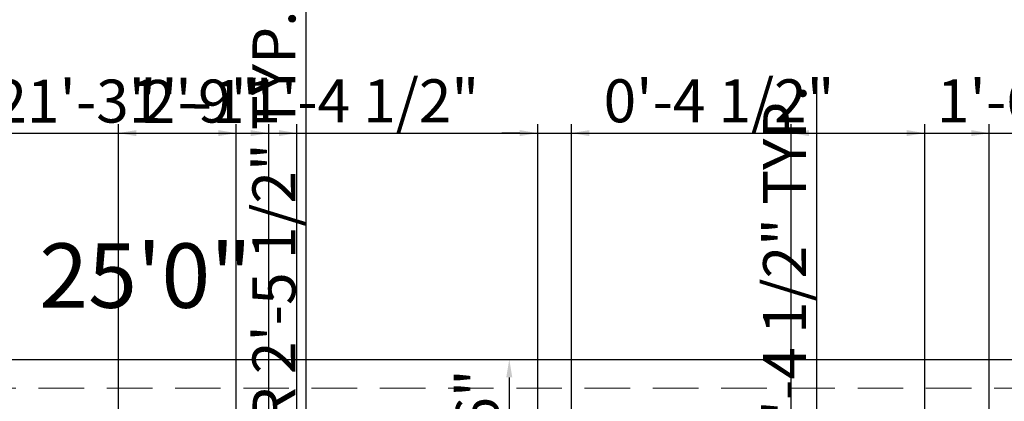
# Model space of a CAD drawing. Units: inches. Extents: x 2656 to 9931, y 1941 to 3068.
# Tile 24 of 46: x 2863 to 3000, y 2636 to 2689. Entities that reach past the tile are written whole.
import ezdxf

# ---------------------------------------------------------------- set-up
doc = ezdxf.new("R2010")
doc.units = ezdxf.units.IN
doc.linetypes.add('DASHED2', pattern=[9.525, 6.35, -3.175])
for name, color, linetype, lineweight in [('A-ANNO-DIMS', 2, 'Continuous', 18), ('A-FLOR-OVHD', 252, 'DASHED2', 13), ('C-PROP', 7, 'Continuous', 25)]:
    doc.layers.add(name, color=color, linetype=linetype, lineweight=lineweight)
doc.styles.get("Standard").update_dxf_attribs({"font": 'arial.ttf'})
doc.dimstyles.new('ISO-25', dxfattribs={"dimtxt": 6, "dimasz": 2.5, "dimexe": 1.25, "dimexo": 0.625, "dimtad": 1, "dimdec": 0, "dimlunit": 3, "dimtxsty": 'Standard', "dimcen": 2.5, "dimadec": 0, "dimazin": 0, "dimtfac": 1, "dimtdec": 0, "dimtmove": 0, "dimatfit": 3, "dimfxl": 1, "dimarcsym": 0})

# ---------------------------------------------------------------- blocks, each defined once
blk = doc.blocks.new('*D2')
at = {"layer": 'A-ANNO-DIMS', "color": 0, "lineweight": -2, "transparency": 16777216}
for p, q in [((2931.82, 2641.6), (2932.44, 2641.6)), ((2931.19, 2639.1), (2931.19, 2626.1)), ((2931.82, 2623.6), (2932.44, 2623.6))]:
    blk.add_line(p, q, dxfattribs=at)
at = {"layer": 'A-ANNO-DIMS', "color": 0, "transparency": 16777216}
for points in [[(2930.77, 2639.1), (2931.61, 2639.1), (2931.19, 2641.6)], [(2930.77, 2626.1), (2931.61, 2626.1), (2931.19, 2623.6)]]:
    blk.add_solid(points, dxfattribs=at)
at = {"layer": 'Defpoints', "color": 0, "transparency": 16777216}
for p in [(2931.19, 2641.6), (2931.19, 2623.6), (2931.19, 2623.6)]:
    blk.add_point(p, dxfattribs=at)
at = {"layer": 'A-ANNO-DIMS', "color": 0, "transparency": 16777216, "insert": (2927.5, 2632.6), "char_height": 6, "attachment_point": 5, "rotation": 90}
blk.add_mtext('1\'6"', dxfattribs=at)
blk = doc.blocks.new('*D33')
at = {"layer": 'A-ANNO-DIMS', "color": 0, "lineweight": -2, "transparency": 16777216}
for p, q in [((2902.86, 2595), (2902.86, 2693.32)), ((2899.03, 2595), (2904.11, 2595)), ((2902.86, 2567.84), (2902.86, 2592.5)), ((2899.03, 2565.34), (2904.11, 2565.34))]:
    blk.add_line(p, q, dxfattribs=at)
at = {"layer": 'A-ANNO-DIMS', "color": 0, "transparency": 16777216}
for points in [[(2902.44, 2592.5), (2903.27, 2592.5), (2902.86, 2595)], [(2902.44, 2567.84), (2903.27, 2567.84), (2902.86, 2565.34)]]:
    blk.add_solid(points, dxfattribs=at)
at = {"layer": 'Defpoints', "color": 0, "transparency": 16777216}
for p in [(2898.41, 2595), (2902.86, 2595), (2898.41, 2565.34)]:
    blk.add_point(p, dxfattribs=at)
at = {"layer": 'A-ANNO-DIMS', "color": 0, "transparency": 16777216, "insert": (2899.13, 2645.41), "char_height": 6, "attachment_point": 5, "rotation": 90}
blk.add_mtext('WC DOOR 2\'-5 1/2" TYP.', dxfattribs=at)
blk = doc.blocks.new('*D45')
at = {"layer": 'A-ANNO-DIMS', "color": 0, "lineweight": -2, "transparency": 16777216}
for p, q in [((2946.51, 2618.48), (2946.51, 2614.25)), ((2970.51, 2618.48), (2970.51, 2614.25)), ((2949.01, 2615.5), (2968.01, 2615.5)), ((2970.51, 2615.5), (3052.06, 2615.5))]:
    blk.add_line(p, q, dxfattribs=at)
at = {"layer": 'A-ANNO-DIMS', "color": 0, "transparency": 16777216}
for points in [[(2949.01, 2615.92), (2949.01, 2615.08), (2946.51, 2615.5)], [(2968.01, 2615.92), (2968.01, 2615.08), (2970.51, 2615.5)]]:
    blk.add_solid(points, dxfattribs=at)
at = {"layer": 'Defpoints', "color": 0, "transparency": 16777216}
for p in [(2946.51, 2619.1), (2970.51, 2619.1), (2970.51, 2615.5)]:
    blk.add_point(p, dxfattribs=at)
at = {"layer": 'A-ANNO-DIMS', "color": 0, "transparency": 16777216, "insert": (3012.54, 2619.23), "char_height": 6, "attachment_point": 5}
blk.add_mtext('WC VENT 2\'-0" TYP.', dxfattribs=at)
blk = doc.blocks.new('*D46')
at = {"layer": 'A-ANNO-DIMS', "color": 0, "lineweight": -2, "transparency": 16777216}
for p, q in [((2974.11, 2626.1), (2974.11, 2680.4)), ((2971.14, 2623.6), (2975.36, 2623.6)), ((2974.11, 2619.1), (2974.11, 2623.6)), ((2971.14, 2619.1), (2975.36, 2619.1)), ((2974.11, 2616.6), (2974.11, 2614.1))]:
    blk.add_line(p, q, dxfattribs=at)
at = {"layer": 'A-ANNO-DIMS', "color": 0, "transparency": 16777216}
for points in [[(2973.7, 2626.1), (2974.53, 2626.1), (2974.11, 2623.6)], [(2973.7, 2616.6), (2974.53, 2616.6), (2974.11, 2619.1)]]:
    blk.add_solid(points, dxfattribs=at)
at = {"layer": 'Defpoints', "color": 0, "transparency": 16777216}
for p in [(2970.51, 2623.6), (2974.11, 2623.6), (2970.51, 2619.1)]:
    blk.add_point(p, dxfattribs=at)
at = {"layer": 'A-ANNO-DIMS', "color": 0, "transparency": 16777216, "insert": (2970.39, 2654.5), "char_height": 6, "attachment_point": 5, "rotation": 90}
blk.add_mtext('0\'-4 1/2" TYP.', dxfattribs=at)
blk = doc.blocks.new('*D57')
at = {"layer": 'A-ANNO-DIMS', "color": 0, "lineweight": -2, "transparency": 16777216}
for p, q in [((2752.16, 2615.23), (2752.16, 2633.85)), ((2872.16, 2615.23), (2872.16, 2633.85)), ((2754.66, 2632.6), (2869.66, 2632.6))]:
    blk.add_line(p, q, dxfattribs=at)
at = {"layer": 'A-ANNO-DIMS', "color": 0, "transparency": 16777216}
for points in [[(2754.66, 2633.02), (2754.66, 2632.18), (2752.16, 2632.6)], [(2869.66, 2633.02), (2869.66, 2632.18), (2872.16, 2632.6)]]:
    blk.add_solid(points, dxfattribs=at)
at = {"layer": 'Defpoints', "color": 0, "transparency": 16777216}
for p in [(2872.16, 2632.6), (2752.16, 2614.6), (2872.16, 2614.6)]:
    blk.add_point(p, dxfattribs=at)
at = {"layer": 'A-ANNO-DIMS', "color": 0, "transparency": 16777216, "insert": (2812.16, 2636.33), "char_height": 6, "attachment_point": 5}
blk.add_mtext('WARDROBE 10\'-0" TYP.', dxfattribs=at)
blk = doc.blocks.new('*D98')
at = {"layer": 'A-ANNO-DIMS', "color": 0, "lineweight": -2, "transparency": 16777216}
for p, q in [((2876.66, 2624.23), (2876.66, 2674.45)), ((2893.09, 2624.23), (2893.09, 2674.45)), ((2879.16, 2673.2), (2890.59, 2673.2)), ((2893.09, 2673.2), (2926.2, 2673.2))]:
    blk.add_line(p, q, dxfattribs=at)
at = {"layer": 'A-ANNO-DIMS', "color": 0, "transparency": 16777216}
for points in [[(2879.16, 2673.62), (2879.16, 2672.78), (2876.66, 2673.2)], [(2890.59, 2673.62), (2890.59, 2672.78), (2893.09, 2673.2)]]:
    blk.add_solid(points, dxfattribs=at)
at = {"layer": 'Defpoints', "color": 0, "transparency": 16777216}
for p in [(2893.09, 2673.2), (2876.66, 2623.6), (2893.09, 2623.6)]:
    blk.add_point(p, dxfattribs=at)
at = {"layer": 'A-ANNO-DIMS', "color": 0, "transparency": 16777216, "insert": (2910.89, 2676.93), "char_height": 6, "attachment_point": 5}
blk.add_mtext('1\'-4 1/2"', dxfattribs=at)
blk = doc.blocks.new('*D99')
at = {"layer": 'A-ANNO-DIMS', "color": 0, "lineweight": -2, "transparency": 16777216}
for p, q in [((2970.51, 2624.23), (2970.51, 2674.45)), ((2989.16, 2624.23), (2989.16, 2674.45)), ((2973.01, 2673.2), (2986.66, 2673.2)), ((2989.16, 2673.2), (3022.27, 2673.2))]:
    blk.add_line(p, q, dxfattribs=at)
at = {"layer": 'A-ANNO-DIMS', "color": 0, "transparency": 16777216}
for points in [[(2973.01, 2673.62), (2973.01, 2672.78), (2970.51, 2673.2)], [(2986.66, 2673.62), (2986.66, 2672.78), (2989.16, 2673.2)]]:
    blk.add_solid(points, dxfattribs=at)
at = {"layer": 'Defpoints', "color": 0, "transparency": 16777216}
for p in [(2989.16, 2673.2), (2970.51, 2623.6), (2989.16, 2623.6)]:
    blk.add_point(p, dxfattribs=at)
at = {"layer": 'A-ANNO-DIMS', "color": 0, "transparency": 16777216, "insert": (3006.97, 2676.93), "char_height": 6, "attachment_point": 5}
blk.add_mtext('1\'-6 1/2"', dxfattribs=at)
blk = doc.blocks.new('*D131')
at = {"layer": 'A-ANNO-DIMS', "color": 0, "lineweight": -2, "transparency": 16777216}
for p, q in [((2876.66, 2539.14), (2876.66, 2674.45)), ((2901.54, 2523.44), (2901.54, 2674.45)), ((2879.16, 2673.2), (2899.04, 2673.2))]:
    blk.add_line(p, q, dxfattribs=at)
at = {"layer": 'A-ANNO-DIMS', "color": 0, "transparency": 16777216}
for points in [[(2879.16, 2673.62), (2879.16, 2672.78), (2876.66, 2673.2)], [(2899.04, 2673.62), (2899.04, 2672.78), (2901.54, 2673.2)]]:
    blk.add_solid(points, dxfattribs=at)
at = {"layer": 'Defpoints', "color": 0, "transparency": 16777216}
for p in [(2901.54, 2673.2), (2876.66, 2538.52), (2901.54, 2522.82)]:
    blk.add_point(p, dxfattribs=at)
at = {"layer": 'A-ANNO-DIMS', "color": 0, "transparency": 16777216, "insert": (2889.1, 2676.84), "char_height": 6, "attachment_point": 5}
blk.add_mtext('2\'-1"', dxfattribs=at)
blk = doc.blocks.new('*D174')
at = {"layer": 'A-ANNO-DIMS', "color": 0, "lineweight": -2, "transparency": 16777216}
for p, q in [((2743.16, 2624.23), (2743.16, 2674.45)), ((2998.16, 2624.23), (2998.16, 2674.45)), ((2745.66, 2673.2), (2995.66, 2673.2))]:
    blk.add_line(p, q, dxfattribs=at)
at = {"layer": 'A-ANNO-DIMS', "color": 0, "transparency": 16777216}
for points in [[(2745.66, 2673.62), (2745.66, 2672.78), (2743.16, 2673.2)], [(2995.66, 2673.62), (2995.66, 2672.78), (2998.16, 2673.2)]]:
    blk.add_solid(points, dxfattribs=at)
at = {"layer": 'Defpoints', "color": 0, "transparency": 16777216}
for p in [(2998.16, 2673.2), (2743.16, 2623.6), (2998.16, 2623.6)]:
    blk.add_point(p, dxfattribs=at)
at = {"layer": 'A-ANNO-DIMS', "color": 0, "transparency": 16777216, "insert": (2870.66, 2676.89), "char_height": 6, "attachment_point": 5}
blk.add_mtext('21\'-3"', dxfattribs=at)
blk = doc.blocks.new('*D176')
at = {"layer": 'A-ANNO-DIMS', "color": 0, "lineweight": -2, "transparency": 16777216}
for p, q in [((2876.66, 2615.23), (2876.66, 2674.45)), ((2897.62, 2615.48), (2897.62, 2674.45)), ((2879.16, 2673.2), (2895.12, 2673.2))]:
    blk.add_line(p, q, dxfattribs=at)
at = {"layer": 'A-ANNO-DIMS', "color": 0, "transparency": 16777216}
for points in [[(2879.16, 2673.62), (2879.16, 2672.78), (2876.66, 2673.2)], [(2895.12, 2673.62), (2895.12, 2672.78), (2897.62, 2673.2)]]:
    blk.add_solid(points, dxfattribs=at)
at = {"layer": 'Defpoints', "color": 0, "transparency": 16777216}
for p in [(2897.62, 2673.2), (2876.66, 2614.6), (2897.62, 2614.86)]:
    blk.add_point(p, dxfattribs=at)
at = {"layer": 'A-ANNO-DIMS', "color": 0, "transparency": 16777216, "insert": (2887.14, 2676.89), "char_height": 6, "attachment_point": 5}
blk.add_mtext('1\'-9"', dxfattribs=at)
blk = doc.blocks.new('*D177')
at = {"layer": 'A-ANNO-DIMS', "color": 0, "lineweight": -2, "transparency": 16777216}
for p, q in [((2935.16, 2615.23), (2935.16, 2674.45)), ((2939.87, 2615.48), (2939.87, 2674.45)), ((2932.66, 2673.2), (2930.16, 2673.2)), ((2935.16, 2673.2), (2939.87, 2673.2)), ((2942.37, 2673.2), (2976.05, 2673.2))]:
    blk.add_line(p, q, dxfattribs=at)
at = {"layer": 'A-ANNO-DIMS', "color": 0, "transparency": 16777216}
for points in [[(2932.66, 2673.62), (2932.66, 2672.78), (2935.16, 2673.2)], [(2942.37, 2673.62), (2942.37, 2672.78), (2939.87, 2673.2)]]:
    blk.add_solid(points, dxfattribs=at)
at = {"layer": 'Defpoints', "color": 0, "transparency": 16777216}
for p in [(2939.87, 2673.2), (2935.16, 2614.6), (2939.87, 2614.86)]:
    blk.add_point(p, dxfattribs=at)
at = {"layer": 'A-ANNO-DIMS', "color": 0, "transparency": 16777216, "insert": (2960.46, 2676.93), "char_height": 6, "attachment_point": 5}
blk.add_mtext('0\'-4 1/2"', dxfattribs=at)
blk = doc.blocks.new('*D190')
at = {"layer": 'A-ANNO-DIMS', "color": 0, "lineweight": -2, "transparency": 16777216}
for p, q in [((2951.95, 2623.98), (2901.83, 2608.18)), ((2890.31, 2604.54), (2899.44, 2607.42))]:
    blk.add_line(p, q, dxfattribs=at)
at = {"layer": 'A-ANNO-DIMS', "color": 0, "transparency": 16777216}
blk.add_solid([(2901.7, 2608.57), (2901.95, 2607.78), (2899.44, 2607.42)], dxfattribs=at)
at = {"layer": 'Defpoints', "color": 0, "transparency": 16777216}
for p in [(2899.44, 2607.42), (2890.31, 2604.54)]:
    blk.add_point(p, dxfattribs=at)
at = {"layer": 'A-ANNO-DIMS', "color": 0, "transparency": 16777216, "insert": (2926.96, 2620.01), "char_height": 6, "attachment_point": 5, "rotation": 17.4987}
blk.add_mtext('4X R0\'-9 1/2"', dxfattribs=at)
blk = doc.blocks.new('*D192')
at = {"layer": 'A-ANNO-DIMS', "color": 0, "lineweight": -2, "transparency": 16777216}
for p, q in [((2848.84, 2626.63), (2897.99, 2608.01)), ((2907.35, 2604.47), (2900.33, 2607.13))]:
    blk.add_line(p, q, dxfattribs=at)
at = {"layer": 'A-ANNO-DIMS', "color": 0, "transparency": 16777216}
blk.add_solid([(2898.14, 2608.4), (2897.84, 2607.62), (2900.33, 2607.13)], dxfattribs=at)
at = {"layer": 'Defpoints', "color": 0, "transparency": 16777216}
for p in [(2900.33, 2607.13), (2907.35, 2604.47)]:
    blk.add_point(p, dxfattribs=at)
at = {"layer": 'A-ANNO-DIMS', "color": 0, "transparency": 16777216, "insert": (2873.57, 2621.25), "char_height": 6, "attachment_point": 5, "rotation": 339.2505}
blk.add_mtext('4X R0\'-7 1/2"', dxfattribs=at)

msp = doc.modelspace()

# ---------------------------------------------------------------- linework, layer by layer
at = {"layer": 'A-FLOR-OVHD'}
msp.add_line((2732.16, 2637.6), (3024.16, 2637.6), dxfattribs=at)
at = {"layer": 'C-PROP'}
msp.add_line((2728.16, 2641.6), (3028.16, 2641.6), dxfattribs=at)

# ---------------------------------------------------------------- texts
at = {"layer": 'A-ANNO-DIMS', "insert": (2865.61, 2657.81), "char_height": 9, "attachment_point": 1}
msp.add_mtext_dynamic_manual_height_columns('25\'0"', width=127.0743, gutter_width=12.5, heights=[0], dxfattribs=at)

# ---------------------------------------------------------------- dimensions: what is measured, and where the dimension line sits
at = {"layer": 'A-ANNO-DIMS'}
for base, p1, p2, text, override, picture, middle in [((2902.86, 2595), (2898.41, 2565.34), (2898.41, 2595), 'WC DOOR <> TYP.', {"dimdec": 1, "dimlfac": 1, "dimrnd": 0, "dimzin": 1, "dimdsep": 46, "dimlunit": 4, "dimfrac": 2}, '*D33', (2899.13, 2645.41)), ((2974.11, 2623.6), (2970.51, 2619.1), (2970.51, 2623.6), '<> TYP.', {"dimdec": 1, "dimlfac": 1, "dimrnd": 0, "dimzin": 1, "dimdsep": 46, "dimlunit": 4, "dimfrac": 2}, '*D46', (2970.39, 2654.5)), ((2931.19, 2623.6), (2931.19, 2641.6), (2931.19, 2623.6), '1\'6"', {"dimclrd": 0, "dimclre": 0, "dimclrt": 0}, '*D2', (2927.5, 2632.6))]:
    dim = msp.add_linear_dim(base=base, p1=p1, p2=p2, angle=90, text=text, dimstyle='ISO-25', override=override, dxfattribs=at)
    dim.commit()
    dim.dimension.update_dxf_attribs({"geometry": picture, "text_midpoint": middle})
for base, p1, p2, picture, middle in [((2893.09, 2673.2), (2876.66, 2623.6), (2893.09, 2623.6), '*D98', (2910.89, 2676.93)), ((2939.87, 2673.2), (2935.16, 2614.6), (2939.87, 2614.86), '*D177', (2960.46, 2676.93)), ((2989.1573, 2673.2003), (2970.5139, 2623.6003), (2989.1573, 2623.6003), '*D99', (3006.9651, 2676.9276)), ((2998.16, 2673.2), (2743.16, 2623.6), (2998.16, 2623.6), '*D174', (2870.66, 2676.89)), ((2897.62, 2673.2), (2876.66, 2614.6), (2897.62, 2614.86), '*D176', (2887.14, 2676.89)), ((2901.54, 2673.2), (2876.66, 2538.52), (2901.54, 2522.82), '*D131', (2889.1, 2676.84))]:
    dim = msp.add_linear_dim(base=base, p1=p1, p2=p2, dimstyle='ISO-25', override={"dimdec": 1, "dimlfac": 1, "dimrnd": 0, "dimzin": 1, "dimdsep": 46, "dimlunit": 4, "dimfrac": 2}, dxfattribs=at)
    dim.commit()
    dim.dimension.update_dxf_attribs({"geometry": picture, "text_midpoint": middle})
for base, p1, p2, text, picture, middle in [((2872.16, 2632.6), (2752.16, 2614.6), (2872.16, 2614.6), 'WARDROBE <> TYP.', '*D57', (2812.16, 2636.33)), ((2970.51, 2615.5), (2946.51, 2619.1), (2970.51, 2619.1), 'WC VENT <> TYP.', '*D45', (3012.54, 2619.23))]:
    dim = msp.add_linear_dim(base=base, p1=p1, p2=p2, text=text, dimstyle='ISO-25', override={"dimdec": 1, "dimlfac": 1, "dimrnd": 0, "dimzin": 1, "dimdsep": 46, "dimlunit": 4, "dimfrac": 2}, dxfattribs=at)
    dim.commit()
    dim.dimension.update_dxf_attribs({"geometry": picture, "text_midpoint": middle})
for center, mpoint, picture, middle in [((2907.35, 2604.47), (2900.33, 2607.13), '*D192', (2873.57, 2621.25)), ((2890.31, 2604.54), (2899.44, 2607.42), '*D190', (2926.96, 2620.01))]:
    dim = msp.add_radius_dim(center=center, mpoint=mpoint, text='4X <>', dimstyle='ISO-25', override={"dimdec": 1, "dimlfac": 1, "dimrnd": 0, "dimzin": 1, "dimdsep": 46, "dimlunit": 4, "dimfrac": 2}, dxfattribs=at)
    dim.commit()
    dim.dimension.update_dxf_attribs({"geometry": picture, "text_midpoint": middle})

doc.saveas('drawing.dxf')
